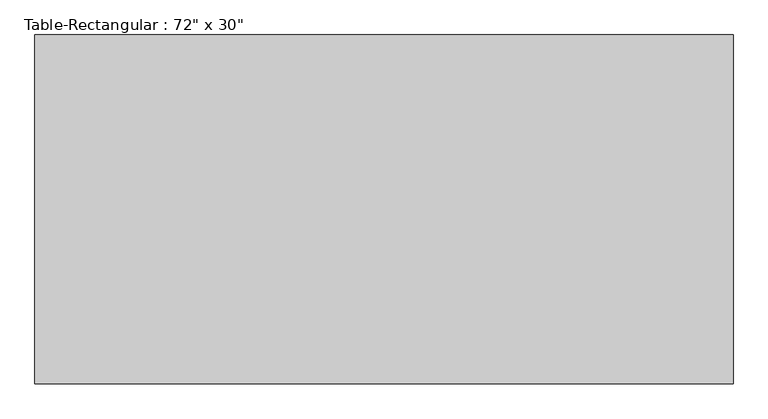
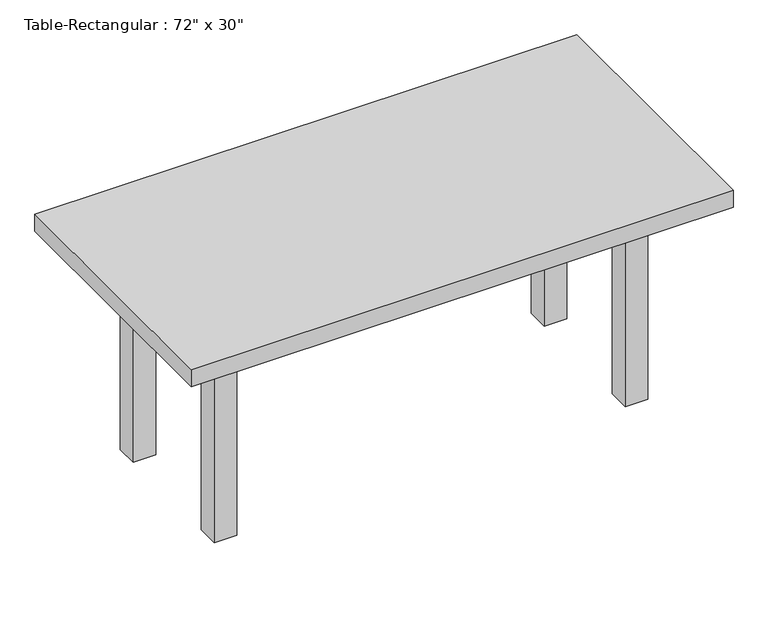
"""IFC4 building model written with IfcOpenShell, lengths in millimetres: furniture geometry."""

from ifc_helpers import new_model, si_unit, frame, origin, origin_with_axes, place, context, project, spatial, polyline, outline, extrude, source, transform, mapped, element, save


def furniture_2bbcfec9(model_context):
    return source(origin(), model_context, "Body", "SweptSolid", [
        extrude(outline(polyline([(546.1, 190.5), (546.1, 165.1), (-546.1, 165.1), (-546.1, 190.5), (546.1, 190.5)])), frame((0.0, 0.0, 508.0), z_axis=(0.0, 0.0, 1.0), x_axis=(1.0, 0.0, 0.0)), (0.0, 0.0, 1.0), 101.6),
        extrude(outline(polyline([(546.1, -190.5), (-546.1, -190.5), (-546.1, -165.1), (546.1, -165.1), (546.1, -190.5)])), frame((0.0, 0.0, 508.0), z_axis=(0.0, 0.0, 1.0), x_axis=(1.0, 0.0, 0.0)), (0.0, 0.0, 1.0), 101.6),
        extrude(outline(polyline([(-558.8, -165.1), (-584.2, -165.1), (-584.2, 165.1), (-558.8, 165.1), (-558.8, -165.1)])), frame((0.0, 0.0, 508.0), z_axis=(0.0, 0.0, 1.0), x_axis=(1.0, 0.0, 0.0)), (0.0, 0.0, 1.0), 101.6),
        extrude(outline(polyline([(558.8, -165.1), (558.8, 165.1), (584.2, 165.1), (584.2, -165.1), (558.8, -165.1)])), frame((0.0, 0.0, 508.0), z_axis=(0.0, 0.0, 1.0), x_axis=(1.0, 0.0, 0.0)), (0.0, 0.0, 1.0), 101.6),
        extrude(outline(polyline([(762.0, 381.0), (762.0, -381.0), (-762.0, -381.0), (-762.0, 381.0), (762.0, 381.0)])), frame((0.0, 0.0, 609.6), z_axis=(0.0, 0.0, 1.0), x_axis=(1.0, 0.0, 0.0)), (0.0, 0.0, 1.0), 50.8),
        extrude(outline(polyline([(-546.1, 228.6), (-546.1, 165.1), (-609.6, 165.1), (-609.6, 228.6), (-546.1, 228.6)])), origin_with_axes(), (0.0, 0.0, 1.0), 609.6),
        extrude(outline(polyline([(546.1, 228.6), (609.6, 228.6), (609.6, 165.1), (546.1, 165.1), (546.1, 228.6)])), origin_with_axes(), (0.0, 0.0, 1.0), 609.6),
        extrude(outline(polyline([(-546.1, -228.6), (-609.6, -228.6), (-609.6, -165.1), (-546.1, -165.1), (-546.1, -228.6)])), origin_with_axes(), (0.0, 0.0, 1.0), 609.6),
        extrude(outline(polyline([(546.1, -228.6), (546.1, -165.1), (609.6, -165.1), (609.6, -228.6), (546.1, -228.6)])), origin_with_axes(), (0.0, 0.0, 1.0), 609.6),
    ])


if __name__ == "__main__":
    model = new_model("IFC4")
    model_context = context("Model", 3, world=origin())
    ifc_project = project(units=[si_unit("LENGTHUNIT", "METRE", prefix="MILLI")], contexts=[model_context])
    site = spatial("IfcSite", under=ifc_project)
    building = spatial("IfcBuilding", under=site)
    placement = place(None, origin())
    furniture_shape = furniture_2bbcfec9(model_context)
    element("IfcFurniture", 1, ObjectType="Table-Rectangular : 72\" x 30\"", at=placement, inside=building, context=model_context, shape_type="MappedRepresentation", body=[
        mapped(furniture_shape, transform((0.0, 0.0, 0.0), x_axis=(1.0, 0.0, 0.0), y_axis=(0.0, 1.0, 0.0), z_axis=(0.0, 0.0, 1.0))),
    ])
    save(model, "model.ifc")

# Revit data of these elements
# Type "Table-Rectangular : 72\" x 30\""
#   Assembly Code = "E2020200"
#   Height = 2' - 2"
#   Length = 5' - 0"
#   Width = 2' - 6"
#   Base Material = Birch
#   Top Material = Birch
#   Default Elevation = 0
# Element 1 (IfcFurniture, "Table-Rectangular : 72\" x 30\"")
#   Materials on its faces: "Birch"
# Materials
#   "Birch": class "Wood", colour RGB 224 178 126, transparency 0, Description = "Betula Alleghaniensis", Cost = 0
